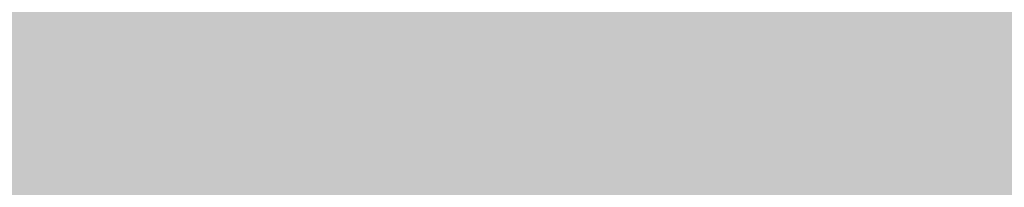
# Model space of a CAD drawing. Units: feet. Extents: x 3168 to 4724, y 827 to 1477.
# Tile 63 of 256: x 3273.147847 to 3273.156253, y 1099.01485 to 1099.016281. Entities that reach past the tile are written whole.
import ezdxf

# ---------------------------------------------------------------- set-up
doc = ezdxf.new("R2010")
doc.units = ezdxf.units.FT
doc.layers.add('A-ELEV', color=7, linetype='Continuous', lineweight=35)
doc.layers.add('A-ELEV-PATT', color=8, linetype='Continuous', lineweight=13)

msp = doc.modelspace()

# ---------------------------------------------------------------- hatches: boundary and pattern name
at = {"layer": 'A-ELEV-PATT'}
h = msp.add_hatch(color=256, dxfattribs=at)
h.dxf.hatch_style = 1
edge = h.paths.add_edge_path()
edge.add_ellipse((3552.9057615, 979.2201412), major_axis=(36.7449243, 0), ratio=0.4848484848, start_angle=0, end_angle=360)
edge = h.paths.add_edge_path()
edge.add_ellipse((3559.8916366, 929.2522824), major_axis=(36.7449243, 0), ratio=0.4848484848, start_angle=0, end_angle=360)
edge = h.paths.add_edge_path()
edge.add_line((3299.3168105, 1198.606081), (3479.9167135, 1198.606081))
edge.add_line((3479.9167135, 1198.606081), (3479.9167135, 1209.8685704))
edge.add_spline(control_points=[(3479.9167135, 1209.8685704), (3464.3011571, 1209.8685704), (3448.6856007, 1209.8685704), (3410.949139, 1209.8685704), (3388.8282339, 1209.8685704), (3355.6468761, 1209.8685704), (3344.5864235, 1209.8685704), (3327.9957446, 1209.8685704), (3322.4655183, 1209.8685704), (3314.1701788, 1209.8685704), (3311.4050657, 1209.8685704), (3307.257396, 1209.8685704), (3305.8748394, 1209.8685704), (3303.8010045, 1209.8685704), (3303.1097262, 1209.8685704), (3302.0728088, 1209.8685704), (3301.7271697, 1209.8685704), (3301.2087109, 1209.8685704), (3301.0358914, 1209.8685704), (3300.776662, 1209.8685704), (3300.6902522, 1209.8685704), (3300.5606376, 1209.8685704), (3300.5174327, 1209.8685704), (3300.4526253, 1209.8685704), (3300.4310229, 1209.8685704), (3300.3986192, 1209.8685704), (3300.387818, 1209.8685704), (3300.3662155, 1209.8685704), (3300.3456757, 1209.8685704), (3300.3455476, 1209.8685704), (3300.345505, 1209.8685704), (3300.3433041, 1209.8685704), (3300.341146, 1209.8685707), (3300.337909, 1209.8685714), (3300.33683, 1209.8685718), (3300.3339422, 1209.8685728), (3300.3321334, 1209.8685736), (3300.3255154, 1209.8685773), (3300.3207065, 1209.8685812), (3300.3109248, 1209.8685917), (3300.305952, 1209.8685984), (3300.2905113, 1209.8686233), (3300.2800452, 1209.8686461), (3300.2324255, 1209.868777), (3300.1952979, 1209.868954), (3299.9510684, 1209.8706077), (3299.7448244, 1209.8743259), (3299.4368271, 1209.8832566), (3299.3343894, 1209.8867924), (3299.181079, 1209.8929197), (3299.1300333, 1209.8950994), (3298.6522171, 1209.9168011), (3298.2294605, 1209.9457176), (3297.6016312, 1210.0023671), (3297.3934043, 1210.0234637), (3297.082652, 1210.058309), (3296.9793324, 1210.0704575), (3296.2929541, 1210.1548606), (3295.7181475, 1210.2433556), (3294.8687167, 1210.3988504), (3294.5876997, 1210.4544779), (3294.1693407, 1210.5433488), (3294.0304153, 1210.5738777), (3291.7071487, 1211.1012), (3289.6535901, 1211.8134353), (3285.7762586, 1213.5639876), (3283.9514101, 1214.6034778), (3280.512159, 1216.9800798), (3278.8972407, 1218.3175918), (3276.3799143, 1220.829489), (3275.4160415, 1221.9177379), (3274.0393421, 1223.7076996), (3273.5810428, 1224.3495346), (3273.1432283, 1225.0163162)], knot_values=[39.119033, 39.119033, 39.119033, 39.119033, 39.286353, 39.286353, 39.523379, 39.523379, 39.641892, 39.641892, 39.701148, 39.701148, 39.730777, 39.730777, 39.745591, 39.745591, 39.752998, 39.752998, 39.756701, 39.756701, 39.758553, 39.758553, 39.759479, 39.759479, 39.759942, 39.759942, 39.760173, 39.760173, 39.760289, 39.760289, 39.760405, 39.760405, 39.760463, 39.760463, 39.763389, 39.763389, 39.764851, 39.764851, 39.767304, 39.767304, 39.773825, 39.773825, 39.78057, 39.78057, 39.79477, 39.79477, 39.845194, 39.845194, 40.126715, 40.126715, 40.267476, 40.267476, 40.337856, 40.337856, 40.927023, 40.927023, 41.221606, 41.221606, 41.368898, 41.368898, 42.202622, 42.202622, 42.619485, 42.619485, 42.827916, 42.827916, 46.118323, 46.118323, 49.408731, 49.408731, 52.699139, 52.699139, 54.927489, 54.927489, 56.104228, 56.104228, 56.104228, 56.104228], weights=[1, 1, 1, 1, 1, 1, 1, 1, 1, 1, 1, 1, 1, 1, 1, 1, 1, 1, 1, 1, 1, 1, 1, 1, 1, 1, 1, 1, 1, 1, 1, 1, 1, 1, 1, 1, 1, 1, 1, 1, 1, 1, 1, 1, 1, 1, 1, 1, 1, 1, 1, 1, 1, 1, 1, 1, 1, 1, 1, 1, 1, 1, 1, 1, 1, 1, 1, 1, 1, 1, 1, 1, 1, 1], degree=3, periodic=0)
edge.add_line((3273.1432283, 1225.0163162), (3273.1432283, 1099.0163162))
edge.add_line((3273.1432283, 1099.0163162), (3299.3168105, 1099.0163162))
edge.add_line((3299.3168105, 1099.0163162), (3299.3168105, 1198.606081))
edge = h.paths.add_edge_path()
edge.add_line((3304.7584434, 1324.15806), (3479.9167135, 1324.15806))
edge.add_line((3479.9167135, 1324.15806), (3479.9167135, 1335.7146184))
edge.add_line((3479.9167135, 1335.7146184), (3269.1616284, 1335.7146184))
edge.add_spline(control_points=[(3269.1616284, 1335.7146184), (3264.0242315, 1335.7146184), (3258.364118, 1328.9581888), (3259.2643109, 1323.9002743)], knot_values=[0, 0, 0, 0, 15.412191, 15.412191, 15.412191, 15.412191], degree=3, periodic=0)
edge.add_line((3259.2643109, 1323.9002743), (3265.5168487, 1288.7691348))
edge.add_line((3265.5168487, 1288.7691348), (3275.2651026, 1261.5456259))
edge.add_line((3275.2651026, 1261.5456259), (3304.7584434, 1261.5456259))
edge.add_line((3304.7584434, 1261.5456259), (3304.7584434, 1324.15806))
h = msp.add_hatch(color=256, dxfattribs=at)
h.dxf.hatch_style = 1
h.paths.add_polyline_path([(3384.5252473, 1099.0163162), (3335.0291678, 1099.0163162), (3299.3168105, 1099.0163162), (3273.1432283, 1099.0163162), (3217.5653642, 1099.0163162), (3168.0692847, 827.1162598), (3335.0291678, 827.1162598)])

# ---------------------------------------------------------------- linework, layer by layer
at = {"layer": 'A-ELEV'}
msp.add_open_spline([(3808.5202001, 1099.0163162), (3808.5202001, 1141.413235), (3808.5202001, 1183.8101539), (3808.5202001, 1226.6353244), (3808.5202001, 1227.0635761), (3808.5202001, 1227.4918279), (3811.491871, 1248.9946729), (3814.463542, 1270.497518), (3817.4652299, 1292.2175635), (3817.4952467, 1292.434764), (3817.5252636, 1292.6519644), (3817.5728014, 1310.1067483), (3817.6203393, 1327.5615322), (3817.6678771, 1345.0163162), (3817.6678771, 1345.4579619), (3817.6678771, 1345.8996077), (3817.6678771, 1346.4560466), (3817.6678771, 1346.5708398), (3817.6678771, 1346.7528874), (3817.6678771, 1346.8201418), (3817.6678771, 1346.9348705), (3817.6678771, 1346.9823447), (3817.6678771, 1347.0385872), (3817.6678771, 1347.0473556), (3817.6678771, 1347.0736607), (3817.667877, 1347.0593025), (3817.6678766, 1347.0615455), (3817.6678764, 1347.0626669), (3817.6678754, 1347.0660311), (3817.6678743, 1347.0682738), (3817.6678701, 1347.0750012), (3817.667866, 1347.0794856), (3817.6678493, 1347.0929368), (3817.6678325, 1347.1019019), (3817.6677657, 1347.1287896), (3817.6676988, 1347.1467049), (3817.6674317, 1347.2004211), (3817.6671649, 1347.2361922), (3817.6661003, 1347.3433849), (3817.6650383, 1347.4146859), (3817.6608124, 1347.6280949), (3817.6566084, 1347.7697085), (3817.6399698, 1348.1924868), (3817.6235091, 1348.4715855), (3817.5590944, 1349.3000666), (3817.4961208, 1349.8405878), (3817.2554319, 1351.4241561), (3817.0263177, 1352.4287852), (3816.3068713, 1354.8889138), (3815.7437452, 1356.2687272), (3814.4639586, 1358.8192105), (3813.7464132, 1359.9909676), (3812.1958378, 1362.1723433), (3811.3622453, 1363.1821237), (3809.5888357, 1365.0690087), (3808.6488164, 1365.9461052), (3806.6542623, 1367.5796162), (3805.5997024, 1368.336154), (3803.3528906, 1369.7223272), (3802.1605354, 1370.352386), (3799.6008131, 1371.4535864), (3798.2326878, 1371.9254812), (3795.2800838, 1372.6346239), (3793.6931479, 1372.8720685), (3791.8694413, 1372.9264797), (3791.7408615, 1372.9292203), (3791.3533713, 1372.9341014), (3791.0927074, 1372.9329013), (3790.3041163, 1372.9150676), (3789.7695426, 1372.8841946), (3789.20919, 1372.8302363), (3789.1906217, 1372.8284241), (3789.1348916, 1372.8229123), (3789.097705, 1372.8191375), (3789.0484446, 1372.8140077), (3789.0364001, 1372.8127432), (3789.0002562, 1372.808918), (3788.9761468, 1372.8063255), (3788.9494049, 1372.8034042), (3788.9467858, 1372.8031177), (3788.9425667, 1372.8026552), (3788.9409669, 1372.8024797), (3788.9385718, 1372.8022166), (3788.9377765, 1372.8021292), (3788.9353908, 1372.8018669), (3788.8675349, 1372.7944024), (3788.7568665, 1372.7822285), (3788.7015323, 1372.7761415), (3788.5355297, 1372.7578805), (3788.4248612, 1372.7457065), (3788.092856, 1372.7091846), (3787.8715192, 1372.6848366), (3787.2075086, 1372.6117927), (3786.764835, 1372.5630968), (3785.436814, 1372.417009), (3784.5514666, 1372.3196171), (3781.8954246, 1372.0274416), (3780.1247299, 1371.8326579), (3774.8126458, 1371.2483067), (3771.2712564, 1370.8587393), (3760.6470883, 1369.6900371), (3753.5643095, 1368.9109022), (3732.3159732, 1366.5734977), (3718.1504157, 1365.015228), (3694.0067577, 1362.3593262), (3684.0286573, 1361.2616941), (3674.0505568, 1360.1640619), (3664.6006617, 1360.1640619), (3655.1507666, 1360.1640619), (3626.8010812, 1360.1640619), (3607.9012909, 1360.1640619), (3551.2019201, 1360.1640619), (3513.4023395, 1360.1640619), (3467.7251817, 1360.1640619), (3459.8476045, 1360.1640619), (3436.2148727, 1360.1640619), (3420.4597182, 1360.1640619), (3373.1942547, 1360.1640619), (3341.6839457, 1360.1640619), (3302.8481616, 1360.1640619), (3295.5226865, 1360.1640619), (3286.0382916, 1360.1640619), (3283.8793719, 1360.1640619), (3277.4026128, 1360.1640619), (3273.0847733, 1360.1640619), (3267.7328511, 1360.1640619), (3266.6987684, 1360.1640619), (3263.5965201, 1360.1640619), (3261.5283546, 1360.1640619), (3259.2369429, 1360.1640619), (3259.0136967, 1360.1640619), (3258.3439582, 1360.1640619), (3257.8974658, 1360.1640619), (3257.4309979, 1360.1640619), (3257.4110224, 1360.1640619), (3257.3705735, 1360.1640619), (3257.3754695, 1360.1640619), (3257.3745975, 1360.1640619), (3257.3739371, 1360.1640618), (3257.3719559, 1360.1640616), (3257.3706351, 1360.1640613), (3257.366673, 1360.16406), (3257.3640318, 1360.1640586), (3257.3561088, 1360.1640529), (3257.3508277, 1360.1640469), (3257.3349869, 1360.1640226), (3257.3244299, 1360.163998), (3257.2927692, 1360.1638987), (3257.2716761, 1360.1637987), (3257.208439, 1360.1633975), (3257.1663373, 1360.1629953), (3257.0402058, 1360.1613882), (3256.9563493, 1360.1597827), (3256.705504, 1360.1533932), (3256.53924, 1360.1470361), (3256.0435702, 1360.1219156), (3255.717296, 1360.0971018), (3254.7524458, 1360.0004808), (3254.1279679, 1359.906513), (3252.1800666, 1359.5253322), (3250.9415739, 1359.1439911), (3248.6701751, 1358.2432905), (3247.6357388, 1357.7238339), (3245.7326321, 1356.6034712), (3244.8633884, 1356.0020595), (3243.2531076, 1354.7428655), (3242.511972, 1354.0847309), (3240.7510518, 1352.3447812), (3239.8009609, 1351.229574), (3238.0877694, 1348.8724402), (3237.3246853, 1347.6303552), (3235.9825098, 1344.9716321), (3235.4022051, 1343.554907), (3234.5910812, 1340.8154577), (3234.3108819, 1339.5435498), (3233.9764902, 1336.8025605), (3233.9221126, 1335.3308771), (3234.1489156, 1332.5912693), (3234.3495287, 1331.3672011), (3234.7198926, 1329.9993668), (3234.7524228, 1329.8833616), (3234.853619, 1329.5347966), (3234.9258923, 1329.301685), (3235.0248359, 1329.0025524), (3235.0469235, 1328.936928), (3235.0776388, 1328.8472393), (3235.0859239, 1328.8231979), (3235.1109389, 1328.7510642), (3235.1278282, 1328.7029624), (3235.1479919, 1328.6462418), (3235.1510592, 1328.6376324), (3235.1560959, 1328.6235265), (3235.1580611, 1328.6180301), (3235.1602094, 1328.6120302), (3235.1656119, 1328.596943), (3235.1800989, 1328.556486), (3235.190263, 1328.5281009), (3235.2207556, 1328.4429457), (3235.241084, 1328.3861755), (3235.3020692, 1328.215865), (3235.3427259, 1328.1023247), (3235.4646962, 1327.7617038), (3235.5460097, 1327.5346232), (3235.7899503, 1326.8533813), (3235.9525774, 1326.39922), (3236.4404586, 1325.0367362), (3236.7657127, 1324.1284137), (3237.7414751, 1321.4034462), (3238.3919833, 1319.5868011), (3240.3435081, 1314.136866), (3241.6445245, 1310.503576), (3245.547574, 1299.6037058), (3248.149607, 1292.3371257), (3255.955706, 1270.5373853), (3261.1597719, 1256.004225), (3267.3876177, 1238.6120011), (3268.4113975, 1235.7529374), (3269.5103781, 1232.6838639), (3269.5855789, 1232.473854), (3269.7066118, 1232.1358507), (3269.752444, 1232.0078573), (3269.8273289, 1231.7987296), (3269.8563817, 1231.7175953), (3269.9063247, 1231.5781217), (3269.927215, 1231.5197823), (3269.9724682, 1231.3934057), (3269.9968311, 1231.3253685), (3270.0265026, 1231.2425062), (3270.0318112, 1231.2276812), (3270.0402823, 1231.2040243), (3270.0392242, 1231.2069792), (3270.0393595, 1231.2066014), (3270.0394271, 1231.2064125), (3270.0396301, 1231.2058458), (3270.0397654, 1231.205468), (3270.0401713, 1231.2043346), (3270.040442, 1231.2035791), (3270.041254, 1231.2013125), (3270.0417955, 1231.1998016), (3270.0434203, 1231.195269), (3270.044504, 1231.1922477), (3270.0477563, 1231.1831849), (3270.0499263, 1231.1771446), (3270.0564418, 1231.1590283), (3270.0607927, 1231.146957), (3270.0738674, 1231.1107614), (3270.0826128, 1231.0866558), (3270.1089357, 1231.0144129), (3270.1265997, 1230.9663498), (3270.1799341, 1230.8224568), (3270.2159467, 1230.7269233), (3270.3253234, 1230.4415078), (3270.4000257, 1230.2528107), (3270.6292491, 1229.6914436), (3270.7888829, 1229.3235005), (3271.2864875, 1228.2383194), (3271.6430996, 1227.5397546), (3272.7758592, 1225.515277), (3273.6141694, 1224.2605021), (3275.4160415, 1221.9177379), (3276.3799143, 1220.829489), (3278.8972407, 1218.3175918), (3280.512159, 1216.9800798), (3283.9514101, 1214.6034778), (3285.7762586, 1213.5639876), (3289.6535901, 1211.8134353), (3291.7071487, 1211.1012), (3294.0304153, 1210.5738777), (3294.1693407, 1210.5433488), (3294.5876997, 1210.4544779), (3294.8687167, 1210.3988504), (3295.7181475, 1210.2433556), (3296.2929541, 1210.1548606), (3296.9793324, 1210.0704575), (3297.082652, 1210.058309), (3297.3934043, 1210.0234637), (3297.6016312, 1210.0023671), (3298.2294605, 1209.9457176), (3298.6522171, 1209.9168011), (3299.1300333, 1209.8950994), (3299.181079, 1209.8929197), (3299.3343894, 1209.8867924), (3299.4368271, 1209.8832566), (3299.7448244, 1209.8743259), (3299.9510684, 1209.8706077), (3300.1952979, 1209.868954), (3300.2324255, 1209.868777), (3300.2800452, 1209.8686461), (3300.2905113, 1209.8686233), (3300.305952, 1209.8685984), (3300.3109248, 1209.8685917), (3300.3207065, 1209.8685812), (3300.3255154, 1209.8685773), (3300.3321334, 1209.8685736), (3300.3339422, 1209.8685728), (3300.33683, 1209.8685718), (3300.337909, 1209.8685714), (3300.341146, 1209.8685707), (3300.3433041, 1209.8685704), (3300.345505, 1209.8685704), (3300.3455476, 1209.8685704), (3300.3456757, 1209.8685704), (3300.3662155, 1209.8685704), (3300.387818, 1209.8685704), (3300.3986192, 1209.8685704), (3300.4310229, 1209.8685704), (3300.4526253, 1209.8685704), (3300.5174327, 1209.8685704), (3300.5606376, 1209.8685704), (3300.6902522, 1209.8685704), (3300.776662, 1209.8685704), (3301.0358914, 1209.8685704), (3301.2087109, 1209.8685704), (3301.7271697, 1209.8685704), (3302.0728088, 1209.8685704), (3303.1097262, 1209.8685704), (3303.8010045, 1209.8685704), (3305.8748394, 1209.8685704), (3307.257396, 1209.8685704), (3311.4050657, 1209.8685704), (3314.1701788, 1209.8685704), (3322.4655183, 1209.8685704), (3327.9957446, 1209.8685704), (3344.5864235, 1209.8685704), (3355.6468761, 1209.8685704), (3388.8282339, 1209.8685704), (3410.949139, 1209.8685704), (3477.3118546, 1209.8685704), (3521.553665, 1209.8685704), (3566.8361836, 1209.8685704), (3567.8768919, 1209.8685704), (3570.9990167, 1209.8685704), (3573.0804332, 1209.8685704), (3575.7813964, 1209.8685704), (3576.4009432, 1209.8685704), (3577.2958211, 1209.8685704), (3577.5711523, 1209.8685704), (3578.3971458, 1209.8685704), (3578.9478081, 1209.8685704), (3579.7564907, 1209.8685704), (3580.0145108, 1209.8685704), (3580.3427367, 1209.8685704), (3580.3268649, 1209.8685704), (3580.3271702, 1209.8685704), (3580.3273229, 1209.8685704), (3580.3277809, 1209.8685704), (3580.3280863, 1209.8685704), (3580.3290024, 1209.8685703), (3580.3296132, 1209.8685702), (3580.3314455, 1209.8685699), (3580.332667, 1209.8685697), (3580.336332, 1209.8685685), (3580.3387755, 1209.8685674), (3580.3461066, 1209.8685629), (3580.350995, 1209.8685584), (3580.3656627, 1209.8685402), (3580.3754446, 1209.868522), (3580.4048012, 1209.8684493), (3580.4243863, 1209.8683764), (3580.4831833, 1209.8680848), (3580.5224371, 1209.8677929), (3580.6403612, 1209.8666242), (3580.7191947, 1209.8654543), (3580.9563152, 1209.8607663), (3581.1152222, 1209.85607), (3581.5941635, 1209.8372298), (3581.9164188, 1209.8183314), (3582.8899466, 1209.7424284), (3583.547986, 1209.6661692), (3585.5318268, 1209.3606172), (3586.8672159, 1209.0538859), (3589.4715454, 1208.2524717), (3590.7402412, 1207.7578521), (3591.9954511, 1207.1588024), (3592.057809, 1207.1287398), (3592.2442418, 1207.0379536), (3592.3676757, 1206.9766317), (3592.73528, 1206.7903591), (3592.9767518, 1206.663101), (3593.2445387, 1206.5164414), (3593.2747313, 1206.4998248), (3593.3651153, 1206.4498388), (3593.4251129, 1206.4163333), (3593.6043138, 1206.3152851), (3593.7227254, 1206.2472105), (3593.8572122, 1206.1683978), (3593.8743621, 1206.1583193), (3593.925741, 1206.1280407), (3593.9598989, 1206.1077976), (3594.0620855, 1206.0468991), (3594.1298272, 1206.0060745), (3594.2084359, 1205.9581709), (3594.2196829, 1205.9513043), (3594.253391, 1205.9306863), (3594.2758193, 1205.9169166), (3594.3429716, 1205.8755358), (3594.3875633, 1205.8478526), (3594.4336161, 1205.8190499), (3594.4352559, 1205.818024), (3594.4401746, 1205.8149461), (3594.4434527, 1205.8128936), (3594.4471229, 1205.8105944), (3594.4475159, 1205.8103482), (3594.4486949, 1205.8096095), (3594.4494808, 1205.8091171), (3594.4503663, 1205.8085621), (3594.4504658, 1205.8084998), (3594.4506003, 1205.8084155), (3594.4673993, 1205.7978872), (3594.4932689, 1205.7816741), (3594.5062037, 1205.7735675), (3594.5450081, 1205.7492479), (3594.5708778, 1205.7330348), (3594.6484866, 1205.6843956), (3594.7002258, 1205.6519694), (3594.8554436, 1205.5546909), (3594.958922, 1205.4898386), (3595.2693574, 1205.2952816), (3595.4763144, 1205.1655769), (3596.0971852, 1204.7764629), (3596.5110991, 1204.5170536), (3597.7528407, 1203.7388256), (3598.5806685, 1203.220007), (3601.0641518, 1201.663551), (3602.7198073, 1200.6259137), (3607.686774, 1197.5130018), (3610.998085, 1195.4377272), (3620.9320182, 1189.2119034), (3627.5546404, 1185.0613542), (3647.4225068, 1172.6097066), (3660.6677511, 1164.3086082), (3700.403484, 1139.405313), (3726.8939725, 1122.8031161), (3757.2057154, 1103.8060516), (3761.0269697, 1101.4111839), (3764.848224, 1099.0163162), (3745.3282713, 1099.0163162), (3725.8083186, 1099.0163162), (3706.288366, 1099.0163162), (3706.288366, 1108.4532371), (3706.288366, 1117.890158), (3706.288366, 1127.3270789), (3710.7507544, 1127.3270789), (3715.2131428, 1127.3270789), (3719.6755312, 1127.3270789)], degree=3, knots=[0, 0, 0, 0, 0.982037, 0.982037, 0.991957, 0.991957, 0.991957, 1.966522, 1.966522, 1.976367, 1.976367, 1.976367, 2.976367, 2.976367, 2.976367, 3.00169, 3.00169, 3.008272, 3.008272, 3.012129, 3.012129, 3.014851, 3.014851, 3.015353, 3.015353, 3.016359, 3.016359, 3.017365, 3.017365, 3.019376, 3.019376, 3.023398, 3.023398, 3.031442, 3.031442, 3.047531, 3.047531, 3.079708, 3.079708, 3.144063, 3.144063, 3.272772, 3.272772, 3.53019, 3.53019, 4.045026, 4.045026, 5.074698, 5.074698, 6.700878, 6.700878, 8.327058, 8.327058, 9.953238, 9.953238, 11.579418, 11.579418, 13.205598, 13.205598, 14.831778, 14.831778, 16.457958, 16.457958, 18.084138, 18.084138, 18.206872, 18.206872, 18.45234, 18.45234, 18.943275, 18.943275, 18.960093, 18.960093, 18.993729, 18.993729, 19.00461, 19.00461, 19.026374, 19.026374, 19.028737, 19.028737, 19.03018, 19.03018, 19.030897, 19.030897, 19.032332, 19.032332, 19.033766, 19.033766, 19.036636, 19.036636, 19.042374, 19.042374, 19.053851, 19.053851, 19.076805, 19.076805, 19.122714, 19.122714, 19.21453, 19.21453, 19.398163, 19.398163, 19.765429, 19.765429, 20.024128, 20.024128, 20.024128, 20.092031, 20.092031, 20.227836, 20.227836, 20.499446, 20.499446, 20.556051, 20.556051, 20.66926, 20.66926, 20.895678, 20.895678, 20.948316, 20.948316, 20.963829, 20.963829, 20.994855, 20.994855, 21.002285, 21.002285, 21.017146, 21.017146, 21.01875, 21.01875, 21.021959, 21.021959, 21.022102, 21.022102, 21.022249, 21.022249, 21.022708, 21.022708, 21.023627, 21.023627, 21.025464, 21.025464, 21.029138, 21.029138, 21.036486, 21.036486, 21.051183, 21.051183, 21.080575, 21.080575, 21.139361, 21.139361, 21.256932, 21.256932, 21.492073, 21.492073, 21.962356, 21.962356, 23.01002, 23.01002, 24.057684, 24.057684, 25.105348, 25.105348, 26.153011, 26.153011, 27.776787, 27.776787, 29.400562, 29.400562, 31.024337, 31.024337, 32.278801, 32.278801, 33.533265, 33.533265, 34.467568, 34.467568, 34.553971, 34.553971, 34.726776, 34.726776, 34.775309, 34.775309, 34.793079, 34.793079, 34.82862, 34.82862, 34.834979, 34.834979, 34.839039, 34.839039, 34.839411, 34.839411, 34.840285, 34.840285, 34.842034, 34.842034, 34.845531, 34.845531, 34.852525, 34.852525, 34.866512, 34.866512, 34.894488, 34.894488, 34.950439, 34.950439, 35.062342, 35.062342, 35.286147, 35.286147, 35.733758, 35.733758, 35.821815, 35.821815, 35.828283, 35.828283, 35.832225, 35.832225, 35.834724, 35.834724, 35.836521, 35.836521, 35.838617, 35.838617, 35.839073, 35.839073, 35.839345, 35.839345, 35.839617, 35.839617, 35.840161, 35.840161, 35.841249, 35.841249, 35.843425, 35.843425, 35.847778, 35.847778, 35.856482, 35.856482, 35.873891, 35.873891, 35.908709, 35.908709, 35.978345, 35.978345, 36.117617, 36.117617, 36.396161, 36.396161, 36.953248, 36.953248, 38.067423, 38.067423, 40.295772, 40.295772, 42.524122, 42.524122, 45.81453, 45.81453, 49.104937, 49.104937, 52.395345, 52.395345, 52.603776, 52.603776, 53.020639, 53.020639, 53.854363, 53.854363, 54.001655, 54.001655, 54.296238, 54.296238, 54.885405, 54.885405, 54.955785, 54.955785, 55.096546, 55.096546, 55.378067, 55.378067, 55.42849, 55.42849, 55.442691, 55.442691, 55.449436, 55.449436, 55.455957, 55.455957, 55.458409, 55.458409, 55.459872, 55.459872, 55.462798, 55.462798, 55.462856, 55.462856, 55.462972, 55.462972, 55.463088, 55.463088, 55.463319, 55.463319, 55.463782, 55.463782, 55.464708, 55.464708, 55.46656, 55.46656, 55.470263, 55.470263, 55.47767, 55.47767, 55.492484, 55.492484, 55.522112, 55.522112, 55.581369, 55.581369, 55.699882, 55.699882, 55.936907, 55.936907, 56.410959, 56.410959, 56.42211, 56.42211, 56.444413, 56.444413, 56.451051, 56.451051, 56.454001, 56.454001, 56.459901, 56.459901, 56.462666, 56.462666, 56.463418, 56.463418, 56.464171, 56.464171, 56.465675, 56.465675, 56.468684, 56.468684, 56.474702, 56.474702, 56.486738, 56.486738, 56.51081, 56.51081, 56.558955, 56.558955, 56.655243, 56.655243, 56.847821, 56.847821, 57.232975, 57.232975, 58.003284, 58.003284, 59.543901, 59.543901, 62.625137, 62.625137, 68.787607, 68.787607, 74.950078, 74.950078, 75.27336, 75.27336, 75.919923, 75.919923, 77.213051, 77.213051, 77.377769, 77.377769, 77.707206, 77.707206, 78.366079, 78.366079, 78.462532, 78.462532, 78.655436, 78.655436, 79.041245, 79.041245, 79.105735, 79.105735, 79.234714, 79.234714, 79.492672, 79.492672, 79.502197, 79.502197, 79.521249, 79.521249, 79.523534, 79.523534, 79.528103, 79.528103, 79.528682, 79.528682, 79.528885, 79.528885, 79.529089, 79.529089, 79.529495, 79.529495, 79.530308, 79.530308, 79.531935, 79.531935, 79.535187, 79.535187, 79.541693, 79.541693, 79.554704, 79.554704, 79.580725, 79.580725, 79.632769, 79.632769, 79.736856, 79.736856, 79.94503, 79.94503, 80.361377, 80.361377, 80.421435, 80.421435, 80.421435, 81.421435, 81.421435, 81.421435, 82.421435, 82.421435, 82.421435, 83.421435, 83.421435, 83.421435, 83.421435], dxfattribs=at)

doc.saveas('drawing.dxf')
